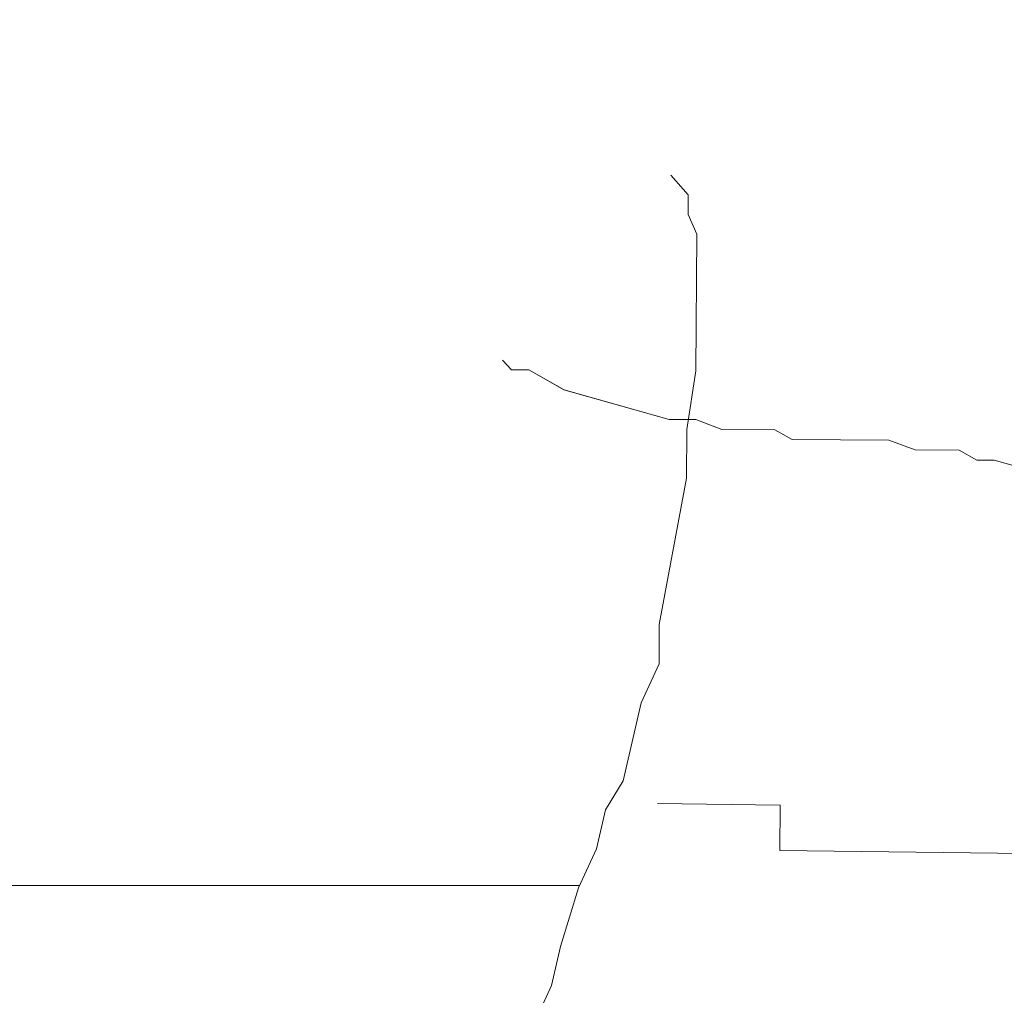
# Model space of a CAD drawing. Units: inches. Extents: x -466983 to 1020, y 324 to 318697.
# Tile 60 of 97: x 631.804 to 634.801, y 945.675 to 948.644. Entities that reach past the tile are written whole.
import ezdxf

# ---------------------------------------------------------------- set-up
doc = ezdxf.new("R2010")
doc.units = ezdxf.units.IN
doc.header["$MEASUREMENT"] = 0
doc.layers.add('A-FLOR-PATT', color=252, linetype='Continuous', lineweight=13)
doc.layers.add('A-FURN', color=8, linetype='Continuous', lineweight=18)

# ---------------------------------------------------------------- blocks, each defined once
blk = doc.blocks.new('L Shaped Sofa')
at = {"ltscale": 2}
for p, q in [((2437.6549, 738.2469), (2437.7044, 738.3551)), ((2437.6048, 738.0303), (2437.6549, 738.2469)), ((2437.5052, 737.7054), (2437.6048, 738.0303)), ((2437.4063, 737.489), (2437.5052, 737.7054)), ((2460.8, 737.6922), (2437.4992, 737.6922)), ((2435.0276, 737.5135), (2436.3886, 737.4969)), ((2436.3886, 737.4969), (2436.3855, 737.245)), ((2437.3562, 737.2724), (2437.4063, 737.489)), ((2436.3855, 737.245), (2437.066, 737.2367)), ((2437.2576, 737.1102), (2437.3562, 737.2724)), ((2437.1573, 736.6769), (2437.2576, 737.1102)), ((2437.0584, 736.4605), (2437.1573, 736.6769)), ((2437.0571, 736.2437), (2437.0584, 736.4605)), ((2436.9057, 735.4311), (2437.0571, 736.2437)), ((2436.9041, 735.16), (2436.9057, 735.4311)), ((2435.0024, 735.3858), (2435.1972, 735.3307)), ((2435.1972, 735.3307), (2435.2948, 735.3302)), ((2435.2948, 735.3302), (2435.3921, 735.2756)), ((2435.3921, 735.2756), (2435.6361, 735.2744)), ((2435.6361, 735.2744), (2435.7821, 735.2195)), ((2435.7821, 735.2195), (2436.3189, 735.217)), ((2436.3189, 735.217), (2436.4161, 735.1623)), ((2436.4161, 735.1623), (2436.7089, 735.1609)), ((2436.7089, 735.1609), (2436.8549, 735.106)), ((2436.8533, 734.835), (2436.9041, 735.16)), ((2436.8549, 735.106), (2437.0013, 735.1054)), ((2437.0013, 735.1054), (2437.5859, 734.94)), ((2437.5859, 734.94), (2437.7804, 734.8306)), ((2436.8486, 734.0759), (2436.8533, 734.835)), ((2437.7804, 734.8306), (2437.878, 734.8302)), ((2437.878, 734.8302), (2437.9264, 734.7757)), ((2436.8968, 733.9673), (2436.8486, 734.0759)), ((2436.8961, 733.8589), (2436.8968, 733.9673)), ((2436.993, 733.75), (2436.8961, 733.8589))]:
    blk.add_line(p, q, dxfattribs=at)

msp = doc.modelspace()

# ---------------------------------------------------------------- hatches: boundary and pattern name
at = {"layer": 'A-FLOR-PATT', "transparency": 33554572}
h = msp.add_hatch(dxfattribs=at)
h.set_pattern_fill('ANSI37', color=256, scale=30)
h.set_pattern_definition([(45, (-1212.4137, -290.035), (-2.6516504, 2.6516504), []), (135, (-1212.4137, -290.035), (-2.6516504, -2.6516504), [])])
h.paths.add_polyline_path([(901.8057, 1075.9377), (900.6144, 1075.9377), (900.6144, 1065.3856), (899.391, 1065.3856), (898.0911, 1065.3856), (892.8356, 1058.7098, -0.258377), (892.1875, 1058.3509), (879.9848, 1058.3509, -0.20177), (879.4382, 1058.5808), (874.0812, 1065.3856), (872.7813, 1065.3856), (871.5579, 1065.3856), (871.5579, 1075.9377), (813.8057, 1075.9377), (813.8057, 1044.7922), (832.3947, 1044.7922, -0.394795), (848.6602, 1028.5356), (848.6602, 1009.9377), (901.8057, 1009.9377), (901.8057, 1015.9377), (901.3057, 1015.9377), (871.3057, 1015.9377), (871.3057, 1017.2502), (871.3344, 1017.2502, -0.401453), (901.3057, 1045.9377), (901.8057, 1045.9377)])
edge = h.paths.add_edge_path(flags=16)
edge.add_line((847.7731, 1068.9486), (847.7731, 1073.7088))
edge.add_arc((849.2269, 1073.7088), 1.4538, 90, 180, ccw=False)
edge.add_line((849.2269, 1075.1627), (864.4921, 1075.1627))
edge.add_arc((864.4921, 1073.7088), 1.4538, 0, 90, ccw=False)
edge.add_line((865.9459, 1073.7088), (865.9459, 1069.0035))
edge.add_arc((832.6447, 1068.9761), 33.3012, -20.61234, 0.04725, ccw=False)
edge.add_ellipse((856.8595, 1058.48), major_axis=(0, 10.2131), ratio=0.6859192, start_angle=100.00884, end_angle=259.99116, ccw=False)
edge.add_arc((881.0742, 1068.9761), 33.3012, 180.04725, 200.61234, ccw=False)
h.paths.add_polyline_path([(853.1456, 1066.4815), (853.1456, 1066.4534), (853.1463, 1066.4534, 0.433107), (852.9166, 1066.6849), (852.9166, 1066.4534), (853.1456, 1066.4534), (853.1456, 1066.4815), (853.088, 1066.6122, 0.697939), (852.6995, 1066.4534), (852.7003, 1066.4534), (852.7003, 1066.4815), (852.9166, 1067.0012), (852.9166, 1066.6849, -0.396254)], flags=0)
h.paths.add_polyline_path([(861.0187, 1066.4815), (861.0187, 1066.4534), (861.0194, 1066.4534, 0.416404), (860.8024, 1066.6849), (860.8024, 1066.4534), (861.0187, 1066.4534), (861.0187, 1066.4815), (860.9672, 1066.6053, 0.713344), (860.5726, 1066.4534), (860.5734, 1066.4534), (860.5734, 1066.4815), (860.8024, 1067.0012), (860.8024, 1066.6849, -0.379973)], flags=0)
edge = h.paths.add_edge_path(flags=0)
edge.add_spline(control_points=[(861.1298, 1065.7855), (861.4661, 1065.2478), (861.6134, 1065.0161), (861.9833, 1064.3736), (862.1924, 1063.9443), (862.5614, 1063.0391), (862.7212, 1062.5633), (862.9865, 1061.5781), (863.092, 1061.0689), (863.2452, 1060.031), (863.293, 1059.5025), (863.3295, 1058.4409), (863.3181, 1057.9078), (863.2366, 1056.8518), (863.1664, 1056.3289), (862.9695, 1055.308), (862.8427, 1054.8099), (862.5365, 1053.8522), (862.3571, 1053.3927), (861.9514, 1052.5249), (861.7251, 1052.1166), (861.233, 1051.3622), (860.9672, 1051.0162), (860.4048, 1050.3949), (860.1082, 1050.1197), (859.4937, 1049.6461), (859.1758, 1049.4476), (858.5276, 1049.1299), (858.1973, 1049.0107), (857.5315, 1048.8518), (857.1959, 1048.8121), (856.5249, 1048.812), (856.1894, 1048.8515), (855.5236, 1049.0101), (855.1933, 1049.1291), (854.545, 1049.4465), (854.2271, 1049.6449), (853.6124, 1050.1183), (853.3158, 1050.3933), (852.7533, 1051.0143), (852.4874, 1051.3602), (851.9952, 1052.1144), (851.7688, 1052.5225), (851.3629, 1053.3902), (851.1834, 1053.8496), (850.877, 1054.8071), (850.7501, 1055.3051), (850.553, 1056.326), (850.4827, 1056.8488), (850.401, 1057.9048), (850.3895, 1058.4379), (850.4257, 1059.4995), (850.4734, 1060.0281), (850.6265, 1061.066), (850.7318, 1061.5753), (850.9969, 1062.5605), (851.1567, 1063.0365), (851.5254, 1063.9418), (851.7345, 1064.3712), (852.1056, 1065.0164), (852.2544, 1065.2503), (852.6082, 1065.7335)], knot_values=[3.915332, 3.915332, 3.915332, 3.915332, 4.013468, 4.013468, 4.175532, 4.175532, 4.337596, 4.337596, 4.49966, 4.49966, 4.661724, 4.661724, 4.823788, 4.823788, 4.985852, 4.985852, 5.147916, 5.147916, 5.30998, 5.30998, 5.472044, 5.472044, 5.634109, 5.634109, 5.796173, 5.796173, 5.958237, 5.958237, 6.120301, 6.120301, 6.282365, 6.282365, 6.444429, 6.444429, 6.606493, 6.606493, 6.768557, 6.768557, 6.930621, 6.930621, 7.092685, 7.092685, 7.254749, 7.254749, 7.416813, 7.416813, 7.578878, 7.578878, 7.740942, 7.740942, 7.903006, 7.903006, 8.06507, 8.06507, 8.227134, 8.227134, 8.389198, 8.389198, 8.551262, 8.551262, 8.65037, 8.65037, 8.65037, 8.65037], degree=3, periodic=0)
edge.add_line((852.6421, 1065.7855), (861.1298, 1065.7855))
edge = h.paths.add_edge_path(flags=0)
edge.add_ellipse((856.8496, 1057.7432), major_axis=(0, 7.7921), ratio=0.687861, start_angle=0, end_angle=360)
h.paths.add_polyline_path([(848.8634, 1069.3891), (848.8634, 1073.9605, -0.414214), (849.9538, 1075.0508), (863.7652, 1075.0508, -0.414214), (864.8555, 1073.9605), (864.8555, 1069.3891, -0.388936), (864.5237, 1069.027, -0.043561), (849.1953, 1069.027, -0.388936)], flags=0)
h.paths.add_polyline_path([(853.1006, 1068.1122, -1), (852.6775, 1068.1122, -1)], flags=0)
edge = h.paths.add_edge_path(flags=0)
edge.add_ellipse((856.8595, 1057.3378), major_axis=(0, 2.207), ratio=0.657164, start_angle=0, end_angle=360)
h.paths.add_polyline_path([(861.0415, 1068.1122, -1), (860.6184, 1068.1122, -1)], flags=0)
edge = h.paths.add_edge_path()
edge.add_line((573.9537, 1057.3412), (573.9537, 1075.9377))
edge.add_line((573.9537, 1075.9377), (558.7308, 1075.9377))
edge.add_line((558.7308, 1075.9377), (558.7308, 1065.3856))
edge.add_line((558.7308, 1065.3856), (557.5074, 1065.3856))
edge.add_line((557.5074, 1065.3856), (556.2075, 1065.3856))
edge.add_line((556.2075, 1065.3856), (550.952, 1058.7098))
edge.add_arc((550.3039, 1059.1155), 0.7646, 270, 327.9483, ccw=False)
edge.add_line((550.3039, 1058.3509), (538.1012, 1058.3509))
edge.add_arc((538.1012, 1059.1155), 0.7646, 224.3704, 270, ccw=False)
edge.add_line((537.5546, 1058.5808), (532.1976, 1065.3856))
edge.add_line((532.1976, 1065.3856), (530.8977, 1065.3856))
edge.add_line((530.8977, 1065.3856), (529.6743, 1065.3856))
edge.add_line((529.6743, 1065.3856), (529.6743, 1075.9377))
edge.add_line((529.6743, 1075.9377), (520.8057, 1075.9377))
edge.add_line((520.8057, 1075.9377), (520.8057, 1045.9377))
edge.add_line((520.8057, 1045.9377), (521.3057, 1045.9377))
edge.add_arc((521.3057, 1015.9377), 30, 2.50749, 90, ccw=False)
edge.add_line((551.277, 1017.2502), (551.3057, 1017.2502))
edge.add_line((551.3057, 1017.2502), (551.3057, 1015.9377))
edge.add_line((551.3057, 1015.9377), (520.8057, 1015.9377))
edge.add_line((520.8057, 1015.9377), (520.8057, 1009.9377))
edge.add_line((520.8057, 1009.9377), (559.1913, 1010.4022))
edge.add_arc((559.1913, 1011.856), 1.4538, 180, 270, ccw=False)
edge.add_line((557.7375, 1011.856), (557.7375, 1016.5613))
edge.add_arc((591.0386, 1016.5888), 33.3012, 159.38766, 180.04725, ccw=False)
edge.add_ellipse((566.8239, 1027.0848), major_axis=(0, 10.2131), ratio=0.6859192, start_angle=280.00884, end_angle=439.99116, ccw=False)
edge.add_arc((542.6091, 1016.5888), 33.3012, 0.04725, 20.61234, ccw=False)
edge.add_line((575.9103, 1016.6162), (575.9103, 1011.856))
edge.add_arc((574.4565, 1011.856), 1.4538, -90, 0, ccw=False)
edge.add_line((574.4565, 1010.4022), (608.8057, 1009.9377))
edge.add_line((608.8057, 1009.9377), (608.8057, 1041.0857))
edge.add_line((608.8057, 1041.0857), (590.2179, 1041.0857))
edge.add_arc((590.775, 1057.9074), 16.8309, 181.92775, 268.10321, ccw=False)
edge = h.paths.add_edge_path()
edge.add_ellipse((494.2443, 583.6204), major_axis=(0, 10.2131), ratio=0.6859192, start_angle=280.00884, end_angle=439.99116, ccw=False)
edge.add_arc((470.0296, 573.1243), 33.3012, 0.04725, 20.61234, ccw=False)
edge.add_line((503.3307, 573.1518), (503.3307, 568.3916))
edge.add_arc((501.8769, 568.3916), 1.4538, -90, 0, ccw=False)
edge.add_line((501.8769, 566.9377), (539.8057, 566.9377))
edge.add_line((539.8057, 566.9377), (539.8057, 572.9377))
edge.add_line((539.8057, 572.9377), (539.3057, 572.9377))
edge.add_line((539.3057, 572.9377), (509.3057, 572.9377))
edge.add_line((509.3057, 572.9377), (509.3057, 574.2502))
edge.add_line((509.3057, 574.2502), (509.3344, 574.2502))
edge.add_arc((539.3057, 572.9377), 30, 90, 177.49251, ccw=False)
edge.add_line((539.3057, 602.9377), (539.8057, 602.9377))
edge.add_line((539.8057, 602.9377), (539.8057, 626.9377))
edge.add_line((539.8057, 626.9377), (531.7718, 626.9377))
edge.add_line((531.7718, 626.9377), (531.7718, 616.3856))
edge.add_line((531.7718, 616.3856), (530.5484, 616.3856))
edge.add_line((530.5484, 616.3856), (529.2485, 616.3856))
edge.add_line((529.2485, 616.3856), (523.7105, 609.3509))
edge.add_line((523.7105, 609.3509), (510.7766, 609.3509))
edge.add_line((510.7766, 609.3509), (505.2386, 616.3856))
edge.add_line((505.2386, 616.3856), (503.9387, 616.3856))
edge.add_line((503.9387, 616.3856), (502.7153, 616.3856))
edge.add_line((502.7153, 616.3856), (502.7153, 626.9377))
edge.add_line((502.7153, 626.9377), (481.6983, 626.9377))
edge.add_line((481.6983, 626.9377), (481.6983, 610.995))
edge.add_arc((467.2703, 611.4728), 14.4359, 271.92775, 358.10321, ccw=False)
edge.add_line((467.7559, 597.0451), (451.8057, 597.0451))
edge.add_line((451.8057, 597.0451), (451.8057, 584.4035))
edge.add_line((451.8057, 584.4035), (451.8057, 566.9377))
edge.add_line((451.8057, 566.9377), (486.6117, 566.9377))
edge.add_arc((486.6117, 568.3916), 1.4538, 180, 270, ccw=False)
edge.add_line((485.1579, 568.3916), (485.1579, 573.0969))
edge.add_arc((518.4591, 573.1243), 33.3012, 159.38766, 180.04725, ccw=False)
h.paths.add_polyline_path([(836.2609, 1020.7328), (879.8898, 1020.7328), (879.8898, 1039.3902), (836.2609, 1039.3902)], flags=25)
h.paths.add_polyline_path([(549.9851, 1036.7492), (593.614, 1036.7492), (593.614, 1055.4065), (549.9851, 1055.4065)], flags=24)
h.paths.add_polyline_path([(475.123, 595.5959), (518.752, 595.5959), (518.752, 614.2532), (475.123, 614.2532)], flags=24)
h = msp.add_hatch(dxfattribs=at)
h.set_pattern_fill('ANSI37', color=256, scale=20)
h.set_pattern_definition([(45, (-1212.4137, -290.035), (-1.767767, 1.767767), []), (135, (-1212.4137, -290.035), (-1.767767, -1.767767), [])])
h.paths.add_polyline_path([(809.8057, 870.9377), (809.8057, 888.1519), (806.9985, 888.1519), (802.6624, 888.1519), (789.3832, 888.1519), (786.2846, 888.1519, -0.414214), (785.4991, 888.9374), (785.4991, 900.1959), (785.4991, 908.4696, -0.414214), (786.8082, 909.7787, -0.414214), (785.4991, 911.0878), (785.4991, 929.1015, -0.414214), (786.8082, 930.4106, -0.414214), (785.4991, 931.7197), (785.4991, 931.9039, -0.414214), (784.19, 930.5948), (766.7223, 930.5948, -0.412359), (765.4132, 931.8956, -0.413741), (764.1145, 930.5782), (744.5781, 930.422, -0.416556), (743.7864, 931.2075), (743.7864, 933.5153), (742.2154, 933.5153), (742.2154, 952.024, -0.001344), (743.7864, 952.1998), (743.7864, 953.9377), (678.5915, 953.9377), (678.5915, 951.1305), (678.5915, 946.7945), (678.5915, 933.5153), (678.5915, 930.4166, -0.414214), (677.806, 929.6312), (666.5475, 929.6312), (658.2738, 929.6312, -0.414214), (656.9647, 930.9403, -0.414214), (655.6556, 929.6312), (637.6419, 929.6312, -0.414214), (636.3328, 930.9403, -0.414214), (635.0237, 929.6312), (634.8395, 929.6312, -0.414214), (636.1486, 928.322), (636.1486, 910.8544, -0.412359), (634.8478, 909.5452, -0.413741), (636.1653, 908.2466), (636.3214, 888.7102, -0.416556), (635.5359, 887.9184), (633.2281, 887.9184), (633.2281, 886.3475), (614.7194, 886.3475, -0.001344), (614.5436, 887.9184), (612.8057, 887.9184), (612.8057, 834.9377), (612.8057, 752.9377), (612.8057, 748.9377), (612.8057, 697.9377), (654.8057, 697.9377), (654.8057, 701.9377), (715.8057, 701.9377), (715.8057, 737.4353), (774.2918, 737.4353), (774.2918, 795.9377), (809.8057, 795.9377)])
h.paths.add_polyline_path([(679.2761, 849.5757, 0.102523), (682.1475, 849.2608, -0.080461), (694.5428, 849.7725, -0.283899), (694.4822, 849.0082, 0.136605), (694.4068, 848.8103, -0.030441), (694.5428, 846.8929), (694.5428, 842.6198), (694.5428, 838.3466, -0.028219), (694.4246, 836.5684), (694.425, 836.5684, 0.196187), (694.4456, 836.2708, -0.302897), (694.5428, 835.467, -0.080461), (682.1475, 835.9787, 0.102523), (679.2761, 835.6638, -0.58611), (678.6457, 836.0169), (678.6457, 849.2227, -0.58611)], flags=16)
h.paths.add_polyline_path([(679.5173, 848.6515, 0.699597), (679.476, 848.6342, 1.20716), (679.1935, 848.7422, 0.010621)], flags=0)
h.paths.add_polyline_path([(679.4923, 836.5608, -0.013798), (679.9178, 836.6594, -0.071703), (682.8533, 837.1434, -0.165743), (682.1665, 839.1006), (682.1665, 842.6094), (682.1665, 846.0603, -0.240616), (683.4733, 848.6767, -0.068263), (693.9295, 849.0082), (693.7875, 848.7083), (693.7875, 849.0228, 0.067332), (683.4733, 848.6767, 0.240616), (682.1665, 846.0603), (682.1665, 842.6094), (682.1665, 839.1006, 0.23459), (683.461, 836.5513, 0.068093), (693.7875, 836.1955), (693.7875, 836.5104), (693.9296, 836.2102, -0.077215), (682.2421, 836.7815, 0.086627), (679.5283, 836.5701, -0.628402), (679.5029, 836.5735), (679.5029, 836.6071, 0.910458)], flags=0)
h.paths.add_polyline_path([(679.476, 848.6364), (679.2069, 848.647), (679.2069, 836.5718, 0.913566), (679.3645, 836.5861), (679.476, 836.5824)], flags=0)
h.paths.add_polyline_path([(679.2761, 829.8604, 0.102523), (682.1475, 829.5455, -0.080461), (694.5428, 830.0572, -0.283899), (694.4822, 829.2929, 0.136605), (694.4068, 829.095, -0.030441), (694.5428, 827.1776), (694.5428, 822.9045), (694.5428, 818.6314, -0.028219), (694.4246, 816.8531), (694.425, 816.8532, 0.196187), (694.4456, 816.5555, -0.302897), (694.5428, 815.7517, -0.080461), (682.1475, 816.2635, 0.102523), (679.2761, 815.9485, -0.58611), (678.6457, 816.3016), (678.6457, 829.5074, -0.58611)], flags=16)
h.paths.add_polyline_path([(679.5173, 828.9362, 0.699597), (679.476, 828.9189, 1.20716), (679.1935, 829.0269, 0.010621)], flags=0)
h.paths.add_polyline_path([(679.4923, 816.8456, -0.013798), (679.9178, 816.9441, -0.071703), (682.8533, 817.4281, -0.165743), (682.1665, 819.3853), (682.1665, 822.8941), (682.1665, 826.345, -0.240616), (683.4733, 828.9614, -0.068263), (693.9295, 829.2929), (693.7875, 828.9931), (693.7875, 829.3076, 0.067332), (683.4733, 828.9614, 0.240616), (682.1665, 826.345), (682.1665, 822.8941), (682.1665, 819.3853, 0.23459), (683.461, 816.836, 0.068093), (693.7875, 816.4802), (693.7875, 816.7952), (693.9296, 816.4949, -0.077215), (682.2421, 817.0662, 0.086627), (679.5283, 816.8549, -0.628402), (679.5029, 816.8582), (679.5029, 816.8918, 0.910458)], flags=0)
h.paths.add_polyline_path([(679.476, 828.9211), (679.2069, 828.9317), (679.2069, 816.8565, 0.913566), (679.3645, 816.8708), (679.476, 816.8671)], flags=0)
h.paths.add_polyline_path([(679.2761, 810.1451, 0.102523), (682.1475, 809.8302, -0.080461), (694.5428, 810.342, -0.3023), (694.4466, 809.5394, 0.10023), (694.4058, 809.3878, -0.03057), (694.5428, 807.4623), (694.5428, 803.1892), (694.5428, 798.9161, -0.03057), (694.4058, 796.9906, 0.10023), (694.4466, 796.839, -0.3023), (694.5428, 796.0365, -0.080461), (682.1475, 796.5482, 0.102523), (679.2761, 796.2333, -0.58611), (678.6457, 796.5863), (678.6457, 809.7921, -0.58611)], flags=16)
h.paths.add_polyline_path([(679.5173, 809.2417, 0.699597), (679.476, 809.2244, 1.20716), (679.1935, 809.3324, 0.010621)], flags=0)
h.paths.add_polyline_path([(679.4923, 797.151, -0.013798), (679.9178, 797.2496, -0.071703), (682.8533, 797.7336, -0.165743), (682.1665, 799.6908), (682.1665, 803.1996), (682.1665, 806.6505, -0.239349), (683.461, 809.2577, -0.072465), (694.4468, 809.5405, 0.197932), (694.425, 809.2405), (693.7875, 809.2985), (693.7875, 809.6135, 0.068093), (683.461, 809.2577, 0.239349), (682.1665, 806.6505), (682.1665, 803.1996), (682.1665, 799.6908, 0.235854), (683.4733, 797.1323, 0.067332), (693.7875, 796.7861), (693.7875, 797.1006), (694.425, 797.1586, 0.197932), (694.4468, 796.8586, -0.080419), (682.1557, 797.3795, 0.083867), (679.5283, 797.1603, -0.628402), (679.5029, 797.1637), (679.5029, 797.1973, 0.910458)], flags=0)
h.paths.add_polyline_path([(679.2069, 809.2372), (679.2069, 797.162, 0.913566), (679.3645, 797.1763), (679.476, 797.1726), (679.476, 809.2266)], flags=0)
h.paths.add_polyline_path([(695.3643, 853.2989), (728.2231, 853.2989), (728.2231, 771.1519), (695.3643, 771.1519)], flags=16)
h.paths.add_polyline_path([(696.0215, 852.6417), (727.5659, 852.6417), (727.5659, 771.809), (696.0215, 771.809)], flags=0)
h.paths.add_polyline_path([(679.2761, 788.7869, 0.102523), (682.1475, 788.472, -0.080461), (694.5428, 788.9837, -0.3023), (694.4466, 788.1812, 0.10023), (694.4058, 788.0296, -0.03057), (694.5428, 786.1041), (694.5428, 781.831), (694.5428, 777.5578, -0.03057), (694.4058, 775.6323, 0.10023), (694.4466, 775.4808, -0.3023), (694.5428, 774.6782, -0.080461), (682.1475, 775.19, 0.102523), (679.2761, 774.875, -0.58611), (678.6457, 775.2281), (678.6457, 788.4339, -0.58611)], flags=16)
h.paths.add_polyline_path([(679.5173, 787.8834, 0.699597), (679.476, 787.8662, 1.20716), (679.1935, 787.9742, 0.010621)], flags=0)
h.paths.add_polyline_path([(679.4923, 775.7928, -0.013798), (679.9178, 775.8914, -0.071703), (682.8533, 776.3753, -0.165743), (682.1665, 778.3325), (682.1665, 781.8414), (682.1665, 785.2922, -0.239349), (683.461, 787.8995, -0.072465), (694.4468, 788.1823, 0.197932), (694.425, 787.8823), (693.7875, 787.9403), (693.7875, 788.2553, 0.068093), (683.461, 787.8995, 0.239349), (682.1665, 785.2922), (682.1665, 781.8414), (682.1665, 778.3325, 0.235854), (683.4733, 775.7741, 0.067332), (693.7875, 775.4279), (693.7875, 775.7424), (694.425, 775.8004, 0.197932), (694.4468, 775.5004, -0.080419), (682.1557, 776.0212, 0.083867), (679.5283, 775.8021, -0.628402), (679.5029, 775.8054), (679.5029, 775.8391, 0.910458)], flags=0)
h.paths.add_polyline_path([(679.2069, 787.8789), (679.2069, 775.8038, 0.913566), (679.3645, 775.818), (679.476, 775.8144), (679.476, 787.8684)], flags=0)
h.paths.add_polyline_path([(704.641, 854.1204, -0.080461), (705.1527, 866.5157, 0.102523), (704.8378, 869.3871, -0.58611), (705.1908, 870.0174), (718.3966, 870.0174, -0.58611), (718.7496, 869.3871, 0.102523), (718.4347, 866.5157, -0.080461), (718.9465, 854.1204, -0.3023), (718.1439, 854.2166, 0.10023), (717.9924, 854.2574, -0.03057), (716.0668, 854.1204), (711.7937, 854.1204), (707.5206, 854.1204, -0.03057), (705.5951, 854.2574, 0.10023), (705.4435, 854.2166, -0.3023)], flags=16)
h.paths.add_polyline_path([(717.8462, 869.1459, 0.699597), (717.8289, 869.1872, 1.20716), (717.9369, 869.4697, 0.010621)], flags=0)
h.paths.add_polyline_path([(705.4631, 854.2164, -0.080419), (705.984, 866.5074, 0.083867), (705.7648, 869.1349, -0.628402), (705.7682, 869.1603), (705.8018, 869.1603, 0.910458), (705.7555, 869.1709, -0.013798), (705.8541, 868.7454, -0.071703), (706.3381, 865.8099, -0.165743), (708.2953, 866.4967), (711.8041, 866.4967), (715.255, 866.4967, -0.239349), (717.8622, 865.2022, -0.072465), (718.145, 854.2164, 0.197932), (717.845, 854.2382), (717.903, 854.8757), (718.218, 854.8757, 0.068093), (717.8622, 865.2022, 0.239349), (715.255, 866.4967), (711.8041, 866.4967), (708.2953, 866.4967, 0.235854), (705.7368, 865.1898, 0.067332), (705.3906, 854.8757), (705.7051, 854.8757), (705.7631, 854.2382, 0.197932)], flags=16)
h.paths.add_polyline_path([(705.7665, 869.4563, 0.913566), (705.7808, 869.2987), (705.7771, 869.1872), (717.8311, 869.1872), (717.8417, 869.4563)], flags=0)
h.paths.add_polyline_path([(729.0446, 842.6198), (729.0446, 846.8929, -0.03057), (729.1817, 848.8184, 0.10023), (729.1408, 848.9699, -0.3023), (729.0446, 849.7725, -0.080461), (741.4399, 849.2608, 0.102523), (744.3113, 849.5757, -0.58611), (744.9417, 849.2227), (744.9417, 836.0169, -0.58611), (744.3113, 835.6638, 0.102523), (741.4399, 835.9787, -0.080461), (729.0446, 835.467, -0.3023), (729.1408, 836.2696, 0.10023), (729.1817, 836.4211, -0.03057), (729.0446, 838.3466)], flags=16)
h.paths.add_polyline_path([(744.1115, 836.5846, 1.20716), (744.3939, 836.4766, 0.010621), (744.0701, 836.5673, 0.699597)], flags=0)
h.paths.add_polyline_path([(729.1407, 836.2684, 0.197932), (729.1624, 836.5684), (729.7999, 836.5104), (729.7999, 836.1955, 0.068093), (740.1264, 836.5513, 0.239349), (741.4209, 839.1585), (741.4209, 842.6094), (741.4209, 846.1182, 0.235854), (740.1141, 848.6767, 0.067332), (729.7999, 849.0228), (729.7999, 848.7083), (729.1624, 848.6503, 0.197932), (729.1407, 848.9504, -0.080419), (741.4317, 848.4295, 0.083867), (744.0591, 848.6486, -0.628402), (744.0845, 848.6453), (744.0845, 848.6117, 0.910458), (744.0951, 848.6579, -0.013798), (743.6696, 848.5594, -0.071703), (740.7341, 848.0754, -0.165743), (741.4209, 846.1182), (741.4209, 842.6094), (741.4209, 839.1585, -0.239349), (740.1264, 836.5513, -0.072465)], flags=0)
h.paths.add_polyline_path([(729.0446, 830.0572, -0.080461), (741.4399, 829.5455, 0.102523), (744.3113, 829.8604, -0.58611), (744.9417, 829.5074), (744.9417, 816.3016, -0.58611), (744.3113, 815.9485, 0.102523), (741.4399, 816.2635, -0.080461), (729.0446, 815.7517, -0.3023), (729.1408, 816.5543, 0.10023), (729.1817, 816.7058, -0.03057), (729.0446, 818.6314), (729.0446, 822.9045), (729.0446, 827.1776, -0.03057), (729.1817, 829.1031, 0.10023), (729.1408, 829.2547, -0.3023)], flags=16)
h.paths.add_polyline_path([(744.1115, 816.8693, 1.20716), (744.3939, 816.7613, 0.010621), (744.0701, 816.852, 0.699597)], flags=0)
h.paths.add_polyline_path([(729.1407, 829.2351, -0.080419), (741.4317, 828.7142, 0.083867), (744.0591, 828.9334, -0.628402), (744.0845, 828.93), (744.0845, 828.8964, 0.910458), (744.0951, 828.9427, -0.013798), (743.6696, 828.8441, -0.071703), (740.7341, 828.3601, -0.165743), (741.4209, 826.4029), (741.4209, 822.8941), (741.4209, 819.4432, -0.239349), (740.1264, 816.836, -0.072465), (729.1407, 816.5531, 0.197932), (729.1624, 816.8532), (729.7999, 816.7952), (729.7999, 816.4802, 0.068093), (740.1264, 816.836, 0.239349), (741.4209, 819.4432), (741.4209, 822.8941), (741.4209, 826.4029, 0.235854), (740.1141, 828.9614, 0.067332), (729.7999, 829.3076), (729.7999, 828.9931), (729.1624, 828.9351, 0.197932)], flags=16)
h.paths.add_polyline_path([(729.0446, 810.342, -0.080461), (741.4399, 809.8302, 0.102523), (744.3113, 810.1451, -0.58611), (744.9417, 809.7921), (744.9417, 796.5863, -0.58611), (744.3113, 796.2333, 0.102523), (741.4399, 796.5482, -0.080461), (729.0446, 796.0365, -0.283899), (729.1052, 796.8007, 0.136605), (729.1806, 796.9987, -0.030441), (729.0446, 798.9161), (729.0446, 803.1892), (729.0446, 807.4623, -0.028219), (729.1628, 809.2406), (729.1624, 809.2405, 0.196187), (729.1418, 809.5382, -0.302897)], flags=16)
h.paths.add_polyline_path([(744.1115, 797.1748, 1.20716), (744.3939, 797.0668, 0.010621), (744.0701, 797.1575, 0.699597)], flags=0)
h.paths.add_polyline_path([(741.3453, 809.0275, 0.086627), (744.0591, 809.2388, -0.628402), (744.0845, 809.2355), (744.0845, 809.2019, 0.910458), (744.0951, 809.2481, -0.013798), (743.6696, 809.1496, -0.071703), (740.7341, 808.6656, -0.165743), (741.4209, 806.7084), (741.4209, 803.1996), (741.4209, 799.7487, -0.240616), (740.1141, 797.1323, -0.068263), (729.658, 796.8008), (729.7999, 797.1006), (729.7999, 796.7861, 0.067332), (740.1141, 797.1323, 0.240616), (741.4209, 799.7487), (741.4209, 803.1996), (741.4209, 806.7084, 0.23459), (740.1264, 809.2577, 0.068093), (729.7999, 809.6135), (729.7999, 809.2985), (729.6578, 809.5988, -0.077215)], flags=0)
h.paths.add_polyline_path([(704.641, 770.3304, -0.283899), (705.4053, 770.2697, 0.136605), (705.6032, 770.1944, -0.030441), (707.5206, 770.3304), (711.7937, 770.3304), (716.0668, 770.3304, -0.028219), (717.8451, 770.2122), (717.845, 770.2126, 0.196187), (718.1427, 770.2331, -0.302897), (718.9465, 770.3304, -0.080461), (718.4347, 757.9351, 0.102523), (718.7496, 755.0637, -0.58611), (718.3966, 754.4333), (705.1908, 754.4333, -0.58611), (704.8378, 755.0637, 0.102523), (705.1527, 757.9351, -0.080461)], flags=16)
h.paths.add_polyline_path([(705.762, 755.3048, 0.699597), (705.7793, 755.2635, 1.20716), (705.6713, 754.9811, 0.010621)], flags=0)
h.paths.add_polyline_path([(705.4053, 769.717), (705.7051, 769.5751), (705.3906, 769.5751, 0.067332), (705.7368, 759.2609, 0.240616), (708.3532, 757.954), (711.8041, 757.954), (715.3129, 757.954, 0.23459), (717.8622, 759.2485, 0.068093), (718.218, 769.5751), (717.903, 769.5751), (718.2033, 769.7172, -0.077215), (717.632, 758.0297, 0.086627), (717.8433, 755.3159, -0.628402), (717.84, 755.2904), (717.8064, 755.2904, 0.910458), (717.8526, 755.2799, -0.013798), (717.7541, 755.7053, -0.071703), (717.2701, 758.6409, -0.165743), (715.3129, 757.954), (711.8041, 757.954), (708.3532, 757.954, -0.240616), (705.7368, 759.2609, -0.068263)], flags=0)
h.paths.add_polyline_path([(729.0446, 788.9837, -0.080461), (741.4399, 788.472, 0.102523), (744.3113, 788.7869, -0.58611), (744.9417, 788.4339), (744.9417, 775.2281, -0.58611), (744.3113, 774.875, 0.102523), (741.4399, 775.19, -0.080461), (729.0446, 774.6782, -0.283899), (729.1052, 775.4425, 0.136605), (729.1806, 775.6405, -0.030441), (729.0446, 777.5578), (729.0446, 781.831), (729.0446, 786.1041, -0.028219), (729.1628, 787.8823), (729.1624, 787.8823, 0.196187), (729.1418, 788.1799, -0.302897)], flags=16)
h.paths.add_polyline_path([(744.1115, 775.8165, 1.20716), (744.3939, 775.7086, 0.010621), (744.0701, 775.7993, 0.699597)], flags=0)
h.paths.add_polyline_path([(741.3453, 787.6692, 0.086627), (744.0591, 787.8806, -0.628402), (744.0845, 787.8773), (744.0845, 787.8437, 0.910458), (744.0951, 787.8899, -0.013798), (743.6696, 787.7913, -0.071703), (740.7341, 787.3074, -0.165743), (741.4209, 785.3502), (741.4209, 781.8414), (741.4209, 778.3905, -0.240616), (740.1141, 775.7741, -0.068263), (729.658, 775.4425), (729.7999, 775.7424), (729.7999, 775.4279, 0.067332), (740.1141, 775.7741, 0.240616), (741.4209, 778.3905), (741.4209, 781.8414), (741.4209, 785.3502, 0.23459), (740.1264, 787.8995, 0.068093), (729.7999, 788.2553), (729.7999, 787.9403), (729.6578, 788.2405, -0.077215)], flags=0)
h.paths.add_polyline_path([(744.1115, 848.6364), (744.1115, 836.5824), (744.3805, 836.5718), (744.3805, 848.647, 0.913566), (744.2229, 848.6327)], flags=0)
h.paths.add_polyline_path([(744.2229, 828.9174), (744.1115, 828.9211), (744.1115, 816.8671), (744.3805, 816.8565), (744.3805, 828.9317, 0.913566)], flags=0)
h.paths.add_polyline_path([(717.8311, 755.2635), (705.7771, 755.2635), (705.7665, 754.9945), (717.8417, 754.9945, 0.913566), (717.8274, 755.1521)], flags=0)
h.paths.add_polyline_path([(744.2229, 809.2229), (744.1115, 809.2266), (744.1115, 797.1726), (744.3805, 797.162), (744.3805, 809.2372, 0.913566)], flags=0)
h.paths.add_polyline_path([(744.1115, 787.8684), (744.1115, 775.8144), (744.3805, 775.8038), (744.3805, 787.8789, 0.913566), (744.2229, 787.8647)], flags=0)
h.paths.add_polyline_path([(678.8774, 877.1228), (737.6127, 877.1228), (737.6127, 899.5116), (678.8774, 899.5116)], flags=24)

# ---------------------------------------------------------------- linework, layer by layer
at = {"layer": 'A-FURN', "ltscale": 2}
for p, q in [((633.7858, 948.1702), (633.8389, 948.1105)), ((633.7858, 948.1702), (633.8389, 948.1105)), ((633.7858, 948.1702), (633.8389, 948.1105)), ((633.7858, 948.1702), (633.8389, 948.1105)), ((633.7858, 948.1702), (633.8389, 948.1105)), ((633.7858, 948.1702), (633.8389, 948.1105)), ((633.8389, 948.1105), (633.8385, 948.0511)), ((633.8389, 948.1105), (633.8385, 948.0511)), ((633.8389, 948.1105), (633.8385, 948.0511)), ((633.8389, 948.1105), (633.8385, 948.0511)), ((633.8389, 948.1105), (633.8385, 948.0511)), ((633.8389, 948.1105), (633.8385, 948.0511)), ((633.8385, 948.0511), (633.8649, 947.9915)), ((633.8385, 948.0511), (633.8649, 947.9915)), ((633.8385, 948.0511), (633.8649, 947.9915)), ((633.8385, 948.0511), (633.8649, 947.9915)), ((633.8385, 948.0511), (633.8649, 947.9915)), ((633.8385, 948.0511), (633.8649, 947.9915)), ((633.8649, 947.9915), (633.8624, 947.5754)), ((633.8649, 947.9915), (633.8624, 947.5754)), ((633.8649, 947.9915), (633.8624, 947.5754)), ((633.8649, 947.9915), (633.8624, 947.5754)), ((633.8649, 947.9915), (633.8624, 947.5754)), ((633.8649, 947.9915), (633.8624, 947.5754)), ((633.3006, 947.578), (633.274, 947.6079)), ((633.3006, 947.578), (633.274, 947.6079)), ((633.3006, 947.578), (633.274, 947.6079)), ((633.3006, 947.578), (633.274, 947.6079)), ((633.3006, 947.578), (633.274, 947.6079)), ((633.3006, 947.578), (633.274, 947.6079)), ((633.3541, 947.5778), (633.3006, 947.578)), ((633.3541, 947.5778), (633.3006, 947.578)), ((633.3541, 947.5778), (633.3006, 947.578)), ((633.3541, 947.5778), (633.3006, 947.578)), ((633.3541, 947.5778), (633.3006, 947.578)), ((633.3541, 947.5778), (633.3006, 947.578)), ((633.4608, 947.5178), (633.3541, 947.5778)), ((633.4608, 947.5178), (633.3541, 947.5778)), ((633.4608, 947.5178), (633.3541, 947.5778)), ((633.4608, 947.5178), (633.3541, 947.5778)), ((633.4608, 947.5178), (633.3541, 947.5778)), ((633.4608, 947.5178), (633.3541, 947.5778)), ((633.8624, 947.5754), (633.8345, 947.3972)), ((633.8624, 947.5754), (633.8345, 947.3972)), ((633.8624, 947.5754), (633.8345, 947.3972)), ((633.8624, 947.5754), (633.8345, 947.3972)), ((633.8624, 947.5754), (633.8345, 947.3972)), ((633.8624, 947.5754), (633.8345, 947.3972)), ((633.7812, 947.4272), (633.4608, 947.5178)), ((633.7812, 947.4272), (633.4608, 947.5178)), ((633.7812, 947.4272), (633.4608, 947.5178)), ((633.7812, 947.4272), (633.4608, 947.5178)), ((633.7812, 947.4272), (633.4608, 947.5178)), ((633.7812, 947.4272), (633.4608, 947.5178)), ((633.8615, 947.4268), (633.7812, 947.4272)), ((633.8615, 947.4268), (633.7812, 947.4272)), ((633.8615, 947.4268), (633.7812, 947.4272)), ((633.8615, 947.4268), (633.7812, 947.4272)), ((633.8615, 947.4268), (633.7812, 947.4272)), ((633.8615, 947.4268), (633.7812, 947.4272)), ((633.9415, 947.3967), (633.8615, 947.4268)), ((633.9415, 947.3967), (633.8615, 947.4268)), ((633.9415, 947.3967), (633.8615, 947.4268)), ((633.9415, 947.3967), (633.8615, 947.4268)), ((633.9415, 947.3967), (633.8615, 947.4268)), ((633.9415, 947.3967), (633.8615, 947.4268)), ((633.8345, 947.3972), (633.8336, 947.2486)), ((633.8345, 947.3972), (633.8336, 947.2486)), ((633.8345, 947.3972), (633.8336, 947.2486)), ((633.8345, 947.3972), (633.8336, 947.2486)), ((633.8345, 947.3972), (633.8336, 947.2486)), ((633.8345, 947.3972), (633.8336, 947.2486)), ((634.102, 947.3959), (633.9415, 947.3967)), ((634.102, 947.3959), (633.9415, 947.3967)), ((634.102, 947.3959), (633.9415, 947.3967)), ((634.102, 947.3959), (633.9415, 947.3967)), ((634.102, 947.3959), (633.9415, 947.3967)), ((634.102, 947.3959), (633.9415, 947.3967)), ((634.1554, 947.366), (634.102, 947.3959)), ((634.1554, 947.366), (634.102, 947.3959)), ((634.1554, 947.366), (634.102, 947.3959)), ((634.1554, 947.366), (634.102, 947.3959)), ((634.1554, 947.366), (634.102, 947.3959)), ((634.1554, 947.366), (634.102, 947.3959)), ((634.4496, 947.3646), (634.1554, 947.366)), ((634.4496, 947.3646), (634.1554, 947.366)), ((634.4496, 947.3646), (634.1554, 947.366)), ((634.4496, 947.3646), (634.1554, 947.366)), ((634.4496, 947.3646), (634.1554, 947.366)), ((634.4496, 947.3646), (634.1554, 947.366)), ((634.5297, 947.3345), (634.4496, 947.3646)), ((634.5297, 947.3345), (634.4496, 947.3646)), ((634.5297, 947.3345), (634.4496, 947.3646)), ((634.5297, 947.3345), (634.4496, 947.3646)), ((634.5297, 947.3345), (634.4496, 947.3646)), ((634.5297, 947.3345), (634.4496, 947.3646)), ((634.6634, 947.3338), (634.5297, 947.3345)), ((634.6634, 947.3338), (634.5297, 947.3345)), ((634.6634, 947.3338), (634.5297, 947.3345)), ((634.6634, 947.3338), (634.5297, 947.3345)), ((634.6634, 947.3338), (634.5297, 947.3345)), ((634.6634, 947.3338), (634.5297, 947.3345)), ((634.7167, 947.3039), (634.6634, 947.3338)), ((634.7167, 947.3039), (634.6634, 947.3338)), ((634.7167, 947.3039), (634.6634, 947.3338)), ((634.7167, 947.3039), (634.6634, 947.3338)), ((634.7167, 947.3039), (634.6634, 947.3338)), ((634.7167, 947.3039), (634.6634, 947.3338)), ((634.7702, 947.3036), (634.7167, 947.3039)), ((634.7702, 947.3036), (634.7167, 947.3039)), ((634.7702, 947.3036), (634.7167, 947.3039)), ((634.7702, 947.3036), (634.7167, 947.3039)), ((634.7702, 947.3036), (634.7167, 947.3039)), ((634.7702, 947.3036), (634.7167, 947.3039)), ((634.8771, 947.2734), (634.7702, 947.3036)), ((634.8771, 947.2734), (634.7702, 947.3036)), ((634.8771, 947.2734), (634.7702, 947.3036)), ((634.8771, 947.2734), (634.7702, 947.3036)), ((634.8771, 947.2734), (634.7702, 947.3036)), ((634.8771, 947.2734), (634.7702, 947.3036)), ((633.8336, 947.2486), (633.7506, 946.8031)), ((633.8336, 947.2486), (633.7506, 946.8031)), ((633.8336, 947.2486), (633.7506, 946.8031)), ((633.8336, 947.2486), (633.7506, 946.8031)), ((633.8336, 947.2486), (633.7506, 946.8031)), ((633.8336, 947.2486), (633.7506, 946.8031)), ((633.7506, 946.8031), (633.7499, 946.6842)), ((633.7506, 946.8031), (633.7499, 946.6842)), ((633.7506, 946.8031), (633.7499, 946.6842)), ((633.7506, 946.8031), (633.7499, 946.6842)), ((633.7506, 946.8031), (633.7499, 946.6842)), ((633.7506, 946.8031), (633.7499, 946.6842)), ((633.7499, 946.6842), (633.6957, 946.5656)), ((633.7499, 946.6842), (633.6957, 946.5656)), ((633.7499, 946.6842), (633.6957, 946.5656)), ((633.7499, 946.6842), (633.6957, 946.5656)), ((633.7499, 946.6842), (633.6957, 946.5656)), ((633.7499, 946.6842), (633.6957, 946.5656)), ((633.6957, 946.5656), (633.6407, 946.3281)), ((633.6957, 946.5656), (633.6407, 946.3281)), ((633.6957, 946.5656), (633.6407, 946.3281)), ((633.6957, 946.5656), (633.6407, 946.3281)), ((633.6957, 946.5656), (633.6407, 946.3281)), ((633.6957, 946.5656), (633.6407, 946.3281)), ((633.6407, 946.3281), (633.5867, 946.2392)), ((633.6407, 946.3281), (633.5867, 946.2392)), ((633.6407, 946.3281), (633.5867, 946.2392)), ((633.6407, 946.3281), (633.5867, 946.2392)), ((633.6407, 946.3281), (633.5867, 946.2392)), ((633.6407, 946.3281), (633.5867, 946.2392)), ((633.5867, 946.2392), (633.5592, 946.1204)), ((633.5867, 946.2392), (633.5592, 946.1204)), ((633.5867, 946.2392), (633.5592, 946.1204)), ((633.5867, 946.2392), (633.5592, 946.1204)), ((633.5867, 946.2392), (633.5592, 946.1204)), ((633.5867, 946.2392), (633.5592, 946.1204)), ((634.1188, 946.2542), (633.7457, 946.2587)), ((634.1188, 946.2542), (633.7457, 946.2587)), ((634.1188, 946.2542), (633.7457, 946.2587)), ((634.1188, 946.2542), (633.7457, 946.2587)), ((634.1188, 946.2542), (633.7457, 946.2587)), ((634.1188, 946.2542), (633.7457, 946.2587)), ((634.1171, 946.1161), (634.1188, 946.2542)), ((634.1171, 946.1161), (634.1188, 946.2542)), ((634.1171, 946.1161), (634.1188, 946.2542)), ((634.1171, 946.1161), (634.1188, 946.2542)), ((634.1171, 946.1161), (634.1188, 946.2542)), ((634.1171, 946.1161), (634.1188, 946.2542)), ((633.5592, 946.1204), (633.505, 946.0018)), ((633.5592, 946.1204), (633.505, 946.0018)), ((633.5592, 946.1204), (633.505, 946.0018)), ((633.5592, 946.1204), (633.505, 946.0018)), ((633.5592, 946.1204), (633.505, 946.0018)), ((633.5592, 946.1204), (633.505, 946.0018)), ((634.8632, 946.1069), (634.1171, 946.1161)), ((634.8632, 946.1069), (634.1171, 946.1161)), ((634.8632, 946.1069), (634.1171, 946.1161)), ((634.8632, 946.1069), (634.1171, 946.1161)), ((634.8632, 946.1069), (634.1171, 946.1161)), ((634.8632, 946.1069), (634.1171, 946.1161)), ((620.7344, 946.009), (633.5083, 946.009)), ((620.7344, 946.009), (633.5083, 946.009)), ((620.7344, 946.009), (633.5083, 946.009)), ((620.7344, 946.009), (633.5083, 946.009)), ((620.7344, 946.009), (633.5083, 946.009)), ((620.7344, 946.009), (633.5083, 946.009)), ((633.505, 946.0018), (633.4504, 945.8237)), ((633.505, 946.0018), (633.4504, 945.8237)), ((633.505, 946.0018), (633.4504, 945.8237)), ((633.505, 946.0018), (633.4504, 945.8237)), ((633.505, 946.0018), (633.4504, 945.8237)), ((633.505, 946.0018), (633.4504, 945.8237)), ((633.4504, 945.8237), (633.4229, 945.7049)), ((633.4504, 945.8237), (633.4229, 945.7049)), ((633.4504, 945.8237), (633.4229, 945.7049)), ((633.4504, 945.8237), (633.4229, 945.7049)), ((633.4504, 945.8237), (633.4229, 945.7049)), ((633.4504, 945.8237), (633.4229, 945.7049)), ((633.4229, 945.7049), (633.3958, 945.6456)), ((633.4229, 945.7049), (633.3958, 945.6456)), ((633.4229, 945.7049), (633.3958, 945.6456)), ((633.4229, 945.7049), (633.3958, 945.6456)), ((633.4229, 945.7049), (633.3958, 945.6456)), ((633.4229, 945.7049), (633.3958, 945.6456))]:
    msp.add_line(p, q, dxfattribs=at)

# ---------------------------------------------------------------- block references
at = {"layer": 'A-FURN', "xscale": 0.5482153745360612, "yscale": 0.5482153745360612, "zscale": 0.5482153745360612, "rotation": 180}
msp.add_blockref('L Shaped Sofa', (1969.7828, 1350.4232), dxfattribs=at)

doc.saveas('drawing.dxf')
